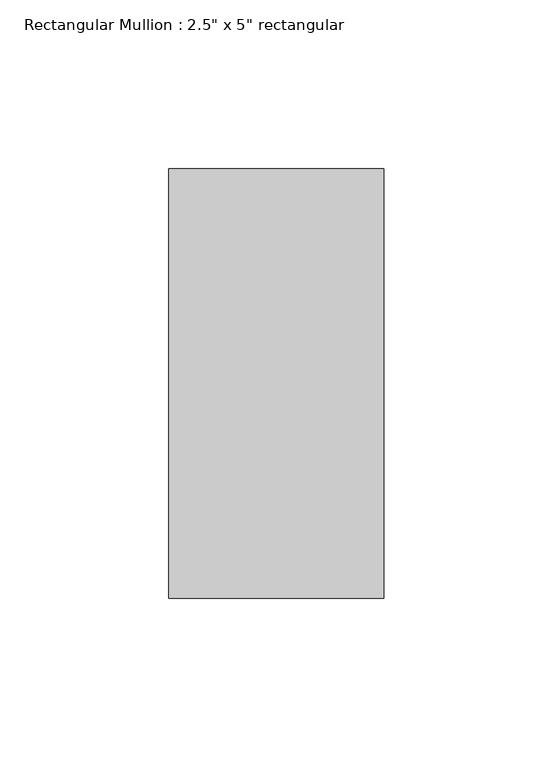
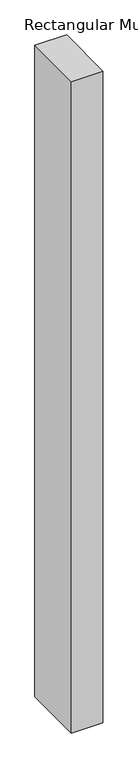
"""IFC4 building model written with IfcOpenShell, lengths in millimetres: member geometry."""

from ifc_helpers import new_model, si_unit, frame, origin, place, context, project, spatial, polyline, outline, extrude, source, transform, mapped, element, save


def member_f7ba7797(model_context):
    return source(origin(), model_context, "Body", "SweptSolid", [
        extrude(outline(polyline([(31.75, 63.5), (31.75, -63.5), (-31.75, -63.5), (-31.75, 63.5), (31.75, 63.5)])), frame((0.0, 0.0, -1384.3), z_axis=(0.0, 0.0, 1.0), x_axis=(1.0, 0.0, 0.0)), (0.0, 0.0, 1.0), 1384.3),
    ])


if __name__ == "__main__":
    model = new_model("IFC4")
    model_context = context("Model", 3, world=origin())
    ifc_project = project(units=[si_unit("LENGTHUNIT", "METRE", prefix="MILLI")], contexts=[model_context])
    site = spatial("IfcSite", under=ifc_project)
    building = spatial("IfcBuilding", under=site)
    placement = place(None, origin())
    member_shape = member_f7ba7797(model_context)
    element("IfcMember", 1, ObjectType="Rectangular Mullion : 2.5\" x 5\" rectangular", at=placement, inside=building, context=model_context, shape_type="MappedRepresentation", body=[
        mapped(member_shape, transform((0.0, 0.0, 0.0), x_axis=(1.0, 0.0, 0.0), y_axis=(0.0, 1.0, 0.0), z_axis=(0.0, 0.0, 1.0))),
    ])
    save(model, "model.ifc")

# Revit data of these elements
# Type "Rectangular Mullion : 2.5\" x 5\" rectangular"
#   built-in parameter 1007304 = 0.416667 (stored number, unit not read)
#   built-in parameter 1007301 = 0.104167 (stored number, unit not read)
#   built-in parameter 1007300 = 0.104167 (stored number, unit not read)
# Element 1 (IfcMember, "Rectangular Mullion : 2.5\" x 5\" rectangular")
#   Materials on its faces: "Aluminum"
# Materials
#   "Aluminum": class "Metal", colour RGB 247 247 247, transparency 0, Description = "Aluminum 6061", Cost = 0
